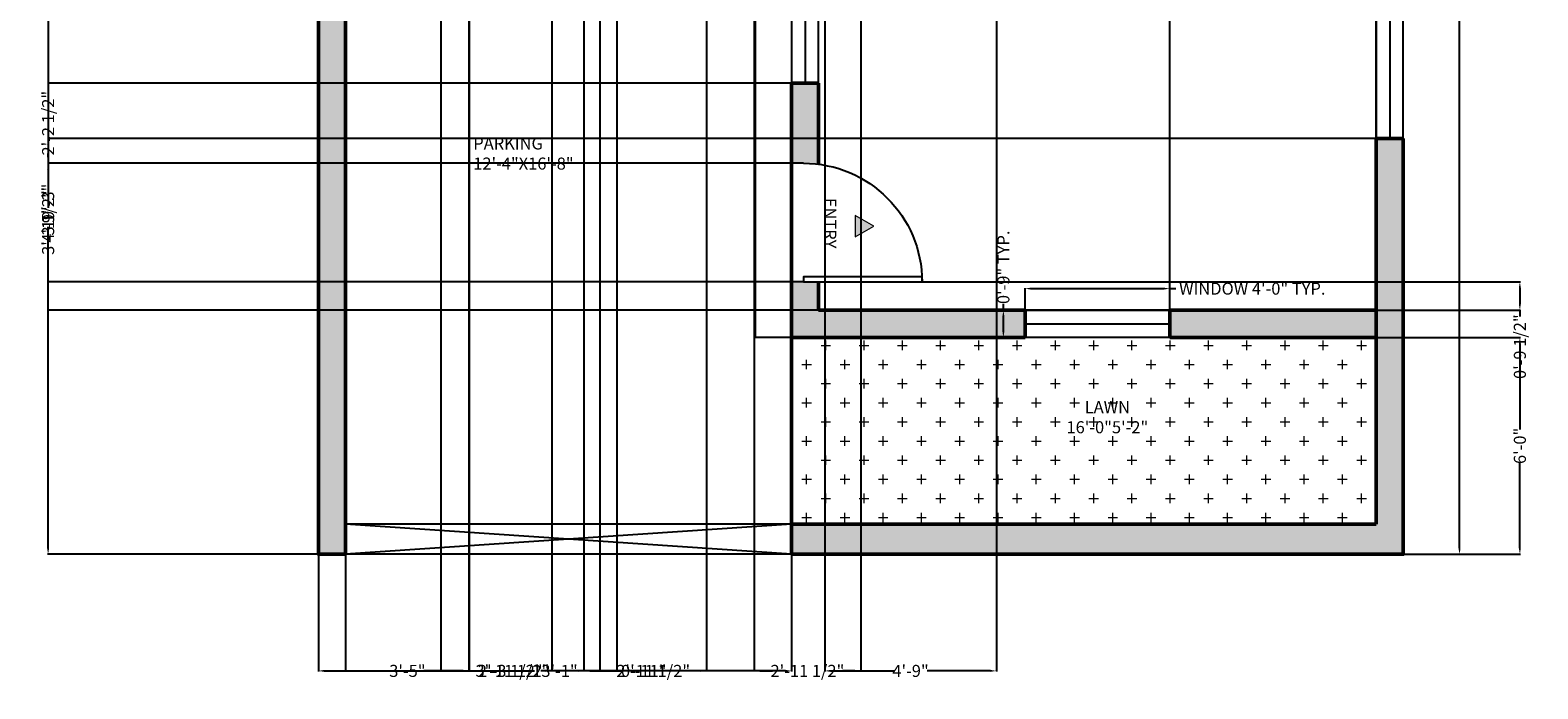
# Model space of a CAD drawing. Units: inches. Extents: x 2430 to 2930, y 1715 to 2575.
# Tile 1 of 4: x 2430 to 2930, y 1715 to 1933. Entities that reach past the tile are written whole.
import ezdxf

# ---------------------------------------------------------------- set-up
doc = ezdxf.new("R2010")
doc.units = ezdxf.units.IN
for name, color, linetype, lineweight in [('A-ANNO-DIMS', 2, 'Continuous', 18), ('A-ANNO-SYMB', 130, 'Continuous', 18), ('A-ANNO-TEXT', 130, 'Continuous', 18), ('A-AREA-IDEN', 130, 'Continuous', 18), ('A-FLOR', 7, 'Continuous', 25), ('A-WALL', 7, 'Continuous', 50), ('A-WALL-PATT', 251, 'Continuous', 13), ('DOOR', 224, 'Continuous', 25), ('L-PLNT-PATT', 116, 'Continuous', 13), ('L-SITE-GATE', 242, 'Continuous', 25), ('win', 170, 'Continuous', 25)]:
    doc.layers.add(name, color=color, linetype=linetype, lineweight=lineweight)
doc.styles.get("Standard").update_dxf_attribs({"font": 'arial.ttf', "height": 4})
doc.dimstyles.get("Standard").update_dxf_attribs({"dimtxt": 4, "dimasz": 2, "dimexe": 0.18, "dimexo": 0.0625, "dimgap": 0.09, "dimtad": 0, "dimzin": 0, "dimdsep": 46, "dimlunit": 3, "dimtxsty": 'Standard', "dimcen": 0.09, "dimadec": 0, "dimazin": 0, "dimtfac": 1, "dimtofl": 0, "dimtmove": 0, "dimatfit": 3, "dimfxl": 1, "dimtolj": 1, "dimtzin": 0, "dimarcsym": 0})

# ---------------------------------------------------------------- blocks, each defined once
blk = doc.blocks.new('*U6')
for p, q in [((0, 0), (0, -100)), ((1000, 0), (1000, -100))]:
    blk.add_line(p, q)
blk.add_lwpolyline([(0, 0), (0, 1000), (43.75, 1000), (43.75, 0)], close=True)
blk.add_arc((0, 0), 1000, 0, 90)
blk = doc.blocks.new('*D12')
at = {"layer": 'A-ANNO-DIMS', "color": 0, "lineweight": -2, "transparency": 16777216}
for p, q in [((2885.68, 2479.45), (2904.48, 2479.45)), ((2904.3, 2477.45), (2904.3, 2122.95)), ((2904.3, 1761.45), (2904.3, 2115.96)), ((2885.68, 1759.45), (2904.48, 1759.45))]:
    blk.add_line(p, q, dxfattribs=at)
at = {"layer": 'A-ANNO-DIMS', "color": 0, "transparency": 16777216}
for points in [[(2903.96, 2477.45), (2904.63, 2477.45), (2904.3, 2479.45)], [(2903.96, 1761.45), (2904.63, 1761.45), (2904.3, 1759.45)]]:
    blk.add_solid(points, dxfattribs=at)
at = {"layer": 'Defpoints', "color": 0, "transparency": 16777216}
for p in [(2885.62, 2479.45), (2885.62, 1759.45), (2904.3, 1759.45)]:
    blk.add_point(p, dxfattribs=at)
at = {"layer": 'A-ANNO-DIMS', "color": 0, "transparency": 16777216, "insert": (2904.3, 2119.45), "char_height": 4, "attachment_point": 5, "rotation": 90}
blk.add_mtext("\\A1;60'", dxfattribs=at)
blk = doc.blocks.new('WIN-48IN')
blk.add_line((0, 4.5), (48, 4.5))
blk.add_lwpolyline([(0, 9), (48, 9), (48, 0), (0, 0)], close=True)
blk = doc.blocks.new('*D17')
at = {"layer": 'A-ANNO-DIMS', "color": 0, "lineweight": -2, "transparency": 16777216}
for p, q in [((2760.12, 1840.52), (2760.12, 1847.83)), ((2762.12, 1847.65), (2806.12, 1847.65)), ((2808.12, 1840.52), (2808.12, 1847.83)), ((2808.12, 1847.65), (2810.12, 1847.65))]:
    blk.add_line(p, q, dxfattribs=at)
at = {"layer": 'A-ANNO-DIMS', "color": 0, "transparency": 16777216}
for points in [[(2762.12, 1847.99), (2762.12, 1847.32), (2760.12, 1847.65)], [(2806.12, 1847.99), (2806.12, 1847.32), (2808.12, 1847.65)]]:
    blk.add_solid(points, dxfattribs=at)
at = {"layer": 'Defpoints', "color": 0, "transparency": 16777216}
for p in [(2808.12, 1847.65), (2760.12, 1840.45), (2808.12, 1840.45)]:
    blk.add_point(p, dxfattribs=at)
at = {"layer": 'A-ANNO-DIMS', "color": 0, "transparency": 16777216, "insert": (2835.52, 1847.65), "char_height": 4, "attachment_point": 5}
blk.add_mtext('\\A1;WINDOW 4\'-0" TYP.', dxfattribs=at)
blk = doc.blocks.new('*D18')
at = {"layer": 'A-ANNO-DIMS', "color": 0, "lineweight": -2, "transparency": 16777216}
for p, q in [((2752.92, 1840.45), (2752.92, 1842.45)), ((2760.06, 1840.45), (2752.74, 1840.45)), ((2752.92, 1833.45), (2752.92, 1838.45)), ((2760.06, 1831.45), (2752.74, 1831.45))]:
    blk.add_line(p, q, dxfattribs=at)
at = {"layer": 'A-ANNO-DIMS', "color": 0, "transparency": 16777216}
for points in [[(2752.59, 1838.45), (2753.25, 1838.45), (2752.92, 1840.45)], [(2752.59, 1833.45), (2753.25, 1833.45), (2752.92, 1831.45)]]:
    blk.add_solid(points, dxfattribs=at)
at = {"layer": 'Defpoints', "color": 0, "transparency": 16777216}
for p in [(2752.92, 1840.45), (2760.12, 1840.45), (2760.12, 1831.45)]:
    blk.add_point(p, dxfattribs=at)
at = {"layer": 'A-ANNO-DIMS', "color": 0, "transparency": 16777216, "insert": (2752.92, 1854.73), "char_height": 4, "attachment_point": 5, "rotation": 90}
blk.add_mtext('\\A1;0\'-9" TYP.', dxfattribs=at)
blk = doc.blocks.new('*D27')
at = {"layer": 'A-ANNO-DIMS', "color": 0, "lineweight": -2, "transparency": 16777216}
for p, q in [((2525.62, 1759.39), (2525.62, 1720.57)), ((2682.62, 1759.39), (2682.62, 1720.57)), ((2527.62, 1720.75), (2597.35, 1720.75)), ((2680.62, 1720.75), (2610.89, 1720.75))]:
    blk.add_line(p, q, dxfattribs=at)
at = {"layer": 'A-ANNO-DIMS', "color": 0, "transparency": 16777216}
for points in [[(2527.62, 1721.09), (2527.62, 1720.42), (2525.62, 1720.75)], [(2680.62, 1721.09), (2680.62, 1720.42), (2682.62, 1720.75)]]:
    blk.add_solid(points, dxfattribs=at)
at = {"layer": 'Defpoints', "color": 0, "transparency": 16777216}
for p in [(2525.62, 1759.45), (2682.62, 1759.45), (2682.62, 1720.75)]:
    blk.add_point(p, dxfattribs=at)
at = {"layer": 'A-ANNO-DIMS', "color": 0, "transparency": 16777216, "insert": (2604.12, 1720.75), "char_height": 4, "attachment_point": 5}
blk.add_mtext('\\A1;13\'-1"', dxfattribs=at)
blk = doc.blocks.new('*D28')
at = {"layer": 'A-ANNO-DIMS', "color": 0, "lineweight": -2, "transparency": 16777216}
for p, q in [((2876.68, 1831.45), (2924.5, 1831.45)), ((2924.32, 1829.45), (2924.32, 1800.87)), ((2924.32, 1761.45), (2924.32, 1790.04)), ((2885.68, 1759.45), (2924.5, 1759.45))]:
    blk.add_line(p, q, dxfattribs=at)
at = {"layer": 'A-ANNO-DIMS', "color": 0, "transparency": 16777216}
for points in [[(2923.99, 1829.45), (2924.65, 1829.45), (2924.32, 1831.45)], [(2923.99, 1761.45), (2924.65, 1761.45), (2924.32, 1759.45)]]:
    blk.add_solid(points, dxfattribs=at)
at = {"layer": 'Defpoints', "color": 0, "transparency": 16777216}
for p in [(2876.62, 1831.45), (2885.62, 1759.45), (2924.32, 1759.45)]:
    blk.add_point(p, dxfattribs=at)
at = {"layer": 'A-ANNO-DIMS', "color": 0, "transparency": 16777216, "insert": (2924.32, 1795.45), "char_height": 4, "attachment_point": 5, "rotation": 90}
blk.add_mtext('\\A1;6\'-0"', dxfattribs=at)
blk = doc.blocks.new('*D29')
at = {"layer": 'A-ANNO-DIMS', "color": 0, "lineweight": -2, "transparency": 16777216}
for p, q in [((2682.56, 1889.27), (2435.74, 1889.27)), ((2435.92, 1887.27), (2435.92, 1879.65)), ((2435.92, 1851.9), (2435.92, 1859.52)), ((2682.56, 1849.9), (2435.74, 1849.9))]:
    blk.add_line(p, q, dxfattribs=at)
at = {"layer": 'A-ANNO-DIMS', "color": 0, "transparency": 16777216}
for points in [[(2435.59, 1887.27), (2436.25, 1887.27), (2435.92, 1889.27)], [(2435.59, 1851.9), (2436.25, 1851.9), (2435.92, 1849.9)]]:
    blk.add_solid(points, dxfattribs=at)
at = {"layer": 'Defpoints', "color": 0, "transparency": 16777216}
for p in [(2435.92, 1889.27), (2682.62, 1889.27), (2682.62, 1849.9)]:
    blk.add_point(p, dxfattribs=at)
at = {"layer": 'A-ANNO-DIMS', "color": 0, "transparency": 16777216, "insert": (2435.92, 1869.58), "char_height": 4, "attachment_point": 5, "rotation": 90}
blk.add_mtext('\\A1;3\'-3 1/2"', dxfattribs=at)
blk = doc.blocks.new('*D30')
at = {"layer": 'A-ANNO-DIMS', "color": 0, "lineweight": -2, "transparency": 16777216}
for p, q in [((2534.62, 2470.39), (2534.62, 1720.57)), ((2575.68, 2470.39), (2575.68, 1720.57)), ((2536.62, 1720.75), (2549.75, 1720.75)), ((2573.68, 1720.75), (2560.56, 1720.75))]:
    blk.add_line(p, q, dxfattribs=at)
at = {"layer": 'A-ANNO-DIMS', "color": 0, "transparency": 16777216}
for points in [[(2536.62, 1721.09), (2536.62, 1720.42), (2534.62, 1720.75)], [(2573.68, 1721.09), (2573.68, 1720.42), (2575.68, 1720.75)]]:
    blk.add_solid(points, dxfattribs=at)
at = {"layer": 'Defpoints', "color": 0, "transparency": 16777216}
for p in [(2534.62, 2470.45), (2575.68, 2470.45), (2575.68, 1720.75)]:
    blk.add_point(p, dxfattribs=at)
at = {"layer": 'A-ANNO-DIMS', "color": 0, "transparency": 16777216, "insert": (2555.15, 1720.75), "char_height": 4, "attachment_point": 5}
blk.add_mtext('\\A1;3\'-5"', dxfattribs=at)
blk = doc.blocks.new('*D34')
at = {"layer": 'A-ANNO-DIMS', "color": 0, "lineweight": -2, "transparency": 16777216}
for p, q in [((2525.56, 1990.45), (2435.74, 1990.45)), ((2435.92, 1988.45), (2435.92, 1881.72)), ((2435.92, 1761.45), (2435.92, 1868.18)), ((2525.56, 1759.45), (2435.74, 1759.45))]:
    blk.add_line(p, q, dxfattribs=at)
at = {"layer": 'A-ANNO-DIMS', "color": 0, "transparency": 16777216}
for points in [[(2435.59, 1988.45), (2436.25, 1988.45), (2435.92, 1990.45)], [(2435.59, 1761.45), (2436.25, 1761.45), (2435.92, 1759.45)]]:
    blk.add_solid(points, dxfattribs=at)
at = {"layer": 'Defpoints', "color": 0, "transparency": 16777216}
for p in [(2435.92, 1990.45), (2525.62, 1990.45), (2525.62, 1759.45)]:
    blk.add_point(p, dxfattribs=at)
at = {"layer": 'A-ANNO-DIMS', "color": 0, "transparency": 16777216, "insert": (2435.92, 1874.95), "char_height": 4, "attachment_point": 5, "rotation": 90}
blk.add_mtext('\\A1;19\'-3"', dxfattribs=at)
blk = doc.blocks.new('*D38')
at = {"layer": 'A-ANNO-DIMS', "color": 0, "lineweight": -2, "transparency": 16777216}
for p, q in [((2876.56, 1897.45), (2435.74, 1897.45)), ((2435.92, 1895.45), (2435.92, 1874.44)), ((2435.92, 1842.45), (2435.92, 1863.47)), ((2876.56, 1840.45), (2435.74, 1840.45))]:
    blk.add_line(p, q, dxfattribs=at)
at = {"layer": 'A-ANNO-DIMS', "color": 0, "transparency": 16777216}
for points in [[(2435.59, 1895.45), (2436.25, 1895.45), (2435.92, 1897.45)], [(2435.59, 1842.45), (2436.25, 1842.45), (2435.92, 1840.45)]]:
    blk.add_solid(points, dxfattribs=at)
at = {"layer": 'Defpoints', "color": 0, "transparency": 16777216}
for p in [(2876.62, 1897.45), (2435.92, 1840.45), (2876.62, 1840.45)]:
    blk.add_point(p, dxfattribs=at)
at = {"layer": 'A-ANNO-DIMS', "color": 0, "transparency": 16777216, "insert": (2435.92, 1868.95), "char_height": 4, "attachment_point": 5, "rotation": 90}
blk.add_mtext('\\A1;4\'-9"', dxfattribs=at)
blk = doc.blocks.new('*D39')
at = {"layer": 'A-ANNO-DIMS', "color": 0, "lineweight": -2, "transparency": 16777216}
for p, q in [((2808.12, 1840.52), (2808.12, 2569.33)), ((2810.12, 2569.15), (2832.3, 2569.15)), ((2874.62, 2569.15), (2852.44, 2569.15)), ((2876.62, 1840.52), (2876.62, 2569.33))]:
    blk.add_line(p, q, dxfattribs=at)
at = {"layer": 'A-ANNO-DIMS', "color": 0, "transparency": 16777216}
for points in [[(2810.12, 2569.49), (2810.12, 2568.82), (2808.12, 2569.15)], [(2874.62, 2569.49), (2874.62, 2568.82), (2876.62, 2569.15)]]:
    blk.add_solid(points, dxfattribs=at)
at = {"layer": 'Defpoints', "color": 0, "transparency": 16777216}
for p in [(2876.62, 2569.15), (2808.12, 1840.45), (2876.62, 1840.45)]:
    blk.add_point(p, dxfattribs=at)
at = {"layer": 'A-ANNO-DIMS', "color": 0, "transparency": 16777216, "insert": (2842.37, 2569.15), "char_height": 4, "attachment_point": 5}
blk.add_mtext('\\A1;5\'-8 1/2"', dxfattribs=at)
blk = doc.blocks.new('*D41')
at = {"layer": 'A-ANNO-DIMS', "color": 0, "lineweight": -2, "transparency": 16777216}
for p, q in [((2693.62, 2062.39), (2693.62, 1720.57)), ((2750.62, 2056.39), (2750.62, 1720.57)), ((2695.62, 1720.75), (2716.63, 1720.75)), ((2748.62, 1720.75), (2727.61, 1720.75))]:
    blk.add_line(p, q, dxfattribs=at)
at = {"layer": 'A-ANNO-DIMS', "color": 0, "transparency": 16777216}
for points in [[(2695.62, 1721.09), (2695.62, 1720.42), (2693.62, 1720.75)], [(2748.62, 1721.09), (2748.62, 1720.42), (2750.62, 1720.75)]]:
    blk.add_solid(points, dxfattribs=at)
at = {"layer": 'Defpoints', "color": 0, "transparency": 16777216}
for p in [(2693.62, 2062.45), (2750.62, 2056.45), (2750.62, 1720.75)]:
    blk.add_point(p, dxfattribs=at)
at = {"layer": 'A-ANNO-DIMS', "color": 0, "transparency": 16777216, "insert": (2722.12, 1720.75), "char_height": 4, "attachment_point": 5}
blk.add_mtext('\\A1;4\'-9"', dxfattribs=at)
blk = doc.blocks.new('*D44')
at = {"layer": 'A-ANNO-DIMS', "color": 0, "lineweight": -2, "transparency": 16777216}
for p, q in [((2670.19, 2218.39), (2670.19, 1720.57)), ((2705.62, 2218.39), (2705.62, 1720.57)), ((2672.19, 1720.75), (2676.25, 1720.75)), ((2703.62, 1720.75), (2699.56, 1720.75))]:
    blk.add_line(p, q, dxfattribs=at)
at = {"layer": 'A-ANNO-DIMS', "color": 0, "transparency": 16777216}
for points in [[(2672.19, 1721.09), (2672.19, 1720.42), (2670.19, 1720.75)], [(2703.62, 1721.09), (2703.62, 1720.42), (2705.62, 1720.75)]]:
    blk.add_solid(points, dxfattribs=at)
at = {"layer": 'Defpoints', "color": 0, "transparency": 16777216}
for p in [(2670.19, 2218.45), (2705.62, 2218.45), (2670.19, 1720.75)]:
    blk.add_point(p, dxfattribs=at)
at = {"layer": 'A-ANNO-DIMS', "color": 0, "transparency": 16777216, "insert": (2687.9, 1720.75), "char_height": 4, "attachment_point": 5}
blk.add_mtext('\\A1;2\'-11 1/2"', dxfattribs=at)
blk = doc.blocks.new('*D45')
at = {"layer": 'A-ANNO-DIMS', "color": 0, "lineweight": -2, "transparency": 16777216}
for p, q in [((2619.01, 2380.39), (2619.01, 1720.57)), ((2654.44, 2380.39), (2654.44, 1720.57)), ((2621.01, 1720.75), (2625.07, 1720.75)), ((2652.44, 1720.75), (2648.38, 1720.75))]:
    blk.add_line(p, q, dxfattribs=at)
at = {"layer": 'A-ANNO-DIMS', "color": 0, "transparency": 16777216}
for points in [[(2621.01, 1721.09), (2621.01, 1720.42), (2619.01, 1720.75)], [(2652.44, 1721.09), (2652.44, 1720.42), (2654.44, 1720.75)]]:
    blk.add_solid(points, dxfattribs=at)
at = {"layer": 'Defpoints', "color": 0, "transparency": 16777216}
for p in [(2619.01, 2380.45), (2654.44, 2380.45), (2654.44, 1720.75)]:
    blk.add_point(p, dxfattribs=at)
at = {"layer": 'A-ANNO-DIMS', "color": 0, "transparency": 16777216, "insert": (2636.72, 1720.75), "char_height": 4, "attachment_point": 5}
blk.add_mtext('\\A1;2\'-11 1/2"', dxfattribs=at)
blk = doc.blocks.new('*D46')
at = {"layer": 'A-ANNO-DIMS', "color": 0, "lineweight": -2, "transparency": 16777216}
for p, q in [((2575.5, 2380.39), (2575.5, 1720.57)), ((2603.06, 2380.39), (2603.06, 1720.57)), ((2577.5, 1720.75), (2579.18, 1720.75)), ((2601.06, 1720.75), (2599.38, 1720.75))]:
    blk.add_line(p, q, dxfattribs=at)
at = {"layer": 'A-ANNO-DIMS', "color": 0, "transparency": 16777216}
for points in [[(2577.5, 1721.09), (2577.5, 1720.42), (2575.5, 1720.75)], [(2601.06, 1721.09), (2601.06, 1720.42), (2603.06, 1720.75)]]:
    blk.add_solid(points, dxfattribs=at)
at = {"layer": 'Defpoints', "color": 0, "transparency": 16777216}
for p in [(2575.5, 2380.45), (2603.06, 2380.45), (2603.06, 1720.75)]:
    blk.add_point(p, dxfattribs=at)
at = {"layer": 'A-ANNO-DIMS', "color": 0, "transparency": 16777216, "insert": (2589.28, 1720.75), "char_height": 4, "attachment_point": 5}
blk.add_mtext('\\A1;2\'-3 1/2"', dxfattribs=at)
blk = doc.blocks.new('*D47')
at = {"layer": 'A-ANNO-DIMS', "color": 0, "lineweight": -2, "transparency": 16777216}
for p, q in [((2682.56, 1915.89), (2435.74, 1915.89)), ((2435.92, 1913.89), (2435.92, 1912.68)), ((2435.92, 1891.27), (2435.92, 1892.48)), ((2682.56, 1889.27), (2435.74, 1889.27))]:
    blk.add_line(p, q, dxfattribs=at)
at = {"layer": 'A-ANNO-DIMS', "color": 0, "transparency": 16777216}
for points in [[(2435.59, 1913.89), (2436.25, 1913.89), (2435.92, 1915.89)], [(2435.59, 1891.27), (2436.25, 1891.27), (2435.92, 1889.27)]]:
    blk.add_solid(points, dxfattribs=at)
at = {"layer": 'Defpoints', "color": 0, "transparency": 16777216}
for p in [(2435.92, 1915.89), (2682.62, 1915.89), (2682.62, 1889.27)]:
    blk.add_point(p, dxfattribs=at)
at = {"layer": 'A-ANNO-DIMS', "color": 0, "transparency": 16777216, "insert": (2435.92, 1902.58), "char_height": 4, "attachment_point": 5, "rotation": 90}
blk.add_mtext('\\A1;2\'-2 1/2"', dxfattribs=at)
blk = doc.blocks.new('*D48')
at = {"layer": 'A-ANNO-DIMS', "color": 0, "lineweight": -2, "transparency": 16777216}
for p, q in [((2691.68, 1849.9), (2924.5, 1849.9)), ((2924.32, 1847.9), (2924.32, 1842.45)), ((2691.68, 1840.45), (2924.5, 1840.45)), ((2924.32, 1840.45), (2924.32, 1838.45))]:
    blk.add_line(p, q, dxfattribs=at)
at = {"layer": 'A-ANNO-DIMS', "color": 0, "transparency": 16777216}
for points in [[(2923.99, 1847.9), (2924.65, 1847.9), (2924.32, 1849.9)], [(2923.99, 1842.45), (2924.65, 1842.45), (2924.32, 1840.45)]]:
    blk.add_solid(points, dxfattribs=at)
at = {"layer": 'Defpoints', "color": 0, "transparency": 16777216}
for p in [(2691.62, 1849.9), (2691.62, 1840.45), (2924.32, 1840.45)]:
    blk.add_point(p, dxfattribs=at)
at = {"layer": 'A-ANNO-DIMS', "color": 0, "transparency": 16777216, "insert": (2924.32, 1828.39), "char_height": 4, "attachment_point": 5, "rotation": 90}
blk.add_mtext('\\A1;0\'-9 1/2"', dxfattribs=at)
blk = doc.blocks.new('*D51')
at = {"layer": 'A-ANNO-DIMS', "color": 0, "lineweight": -2, "transparency": 16777216}
for p, q in [((2566.24, 2197.83), (2566.24, 1720.57)), ((2613.75, 2197.83), (2613.75, 1720.57)), ((2568.24, 1720.75), (2578.38, 1720.75)), ((2611.75, 1720.75), (2601.62, 1720.75))]:
    blk.add_line(p, q, dxfattribs=at)
at = {"layer": 'A-ANNO-DIMS', "color": 0, "transparency": 16777216}
for points in [[(2568.24, 1721.09), (2568.24, 1720.42), (2566.24, 1720.75)], [(2611.75, 1721.09), (2611.75, 1720.42), (2613.75, 1720.75)]]:
    blk.add_solid(points, dxfattribs=at)
at = {"layer": 'Defpoints', "color": 0, "transparency": 16777216}
for p in [(2566.24, 2197.89), (2613.75, 2197.89), (2613.75, 1720.75)]:
    blk.add_point(p, dxfattribs=at)
at = {"layer": 'A-ANNO-DIMS', "color": 0, "transparency": 16777216, "insert": (2590, 1720.75), "char_height": 4, "attachment_point": 5}
blk.add_mtext('\\A1;3\'-11 1/2"', dxfattribs=at)
blk = doc.blocks.new('*D53')
at = {"layer": 'A-ANNO-DIMS', "color": 0, "lineweight": -2, "transparency": 16777216}
for p, q in [((2613.75, 2197.83), (2613.75, 1720.57)), ((2624.62, 2194.39), (2624.62, 1720.57)), ((2615.75, 1720.75), (2622.62, 1720.75)), ((2624.62, 1720.75), (2626.62, 1720.75))]:
    blk.add_line(p, q, dxfattribs=at)
at = {"layer": 'A-ANNO-DIMS', "color": 0, "transparency": 16777216}
for points in [[(2615.75, 1721.09), (2615.75, 1720.42), (2613.75, 1720.75)], [(2622.62, 1721.09), (2622.62, 1720.42), (2624.62, 1720.75)]]:
    blk.add_solid(points, dxfattribs=at)
at = {"layer": 'Defpoints', "color": 0, "transparency": 16777216}
for p in [(2613.75, 2197.89), (2624.62, 2194.45), (2624.62, 1720.75)]:
    blk.add_point(p, dxfattribs=at)
at = {"layer": 'A-ANNO-DIMS', "color": 0, "transparency": 16777216, "insert": (2633.58, 1720.75), "char_height": 4, "attachment_point": 5}
blk.add_mtext('\\A1;0\'-11"', dxfattribs=at)

msp = doc.modelspace()

# ---------------------------------------------------------------- hatches: boundary and pattern name
at = {"layer": 'A-ANNO-SYMB'}
h = msp.add_hatch(color=256, dxfattribs=at)
h.dxf.hatch_style = 1
h.paths.add_polyline_path([(2709.881, 1868.357), (2703.752, 1871.895), (2703.752, 1864.818)])
at = {"layer": 'A-WALL-PATT'}
h = msp.add_hatch(color=256, dxfattribs=at)
h.dxf.hatch_style = 1
h.paths.add_polyline_path([(2885.621, 1897.453), (2876.621, 1897.453), (2876.621, 1769.453), (2682.621, 1769.453), (2682.621, 1759.453), (2885.621, 1759.453)])
h.paths.add_polyline_path([(2885.621, 2020.453), (2876.621, 2020.453), (2876.621, 1945.453), (2885.621, 1945.453)])
h.paths.add_polyline_path([(2876.621, 1840.453), (2808.121, 1840.453), (2808.121, 1831.453), (2876.621, 1831.453)], flags=17)
h.paths.add_polyline_path([(2760.121, 1840.453), (2691.621, 1840.453), (2691.621, 1849.896), (2686.558, 1849.896), (2682.621, 1849.896), (2682.621, 1831.453), (2760.121, 1831.453)], flags=17)
h.paths.add_polyline_path([(2691.621, 1915.889), (2682.621, 1915.889), (2682.621, 1889.266), (2686.558, 1889.266, -0.0322505), (2691.621, 1888.939)])
h.paths.add_polyline_path([(2691.621, 2056.453), (2693.621, 2056.453), (2693.621, 2062.453), (2682.621, 2062.453), (2677.568, 2062.453), (2677.568, 2057.39), (2677.568, 2053.453), (2682.621, 2053.453), (2682.621, 1975.453), (2673.244, 1975.453), (2673.244, 1970.39), (2673.244, 1966.453), (2682.621, 1966.453), (2682.621, 1963.889), (2691.621, 1963.889)])
h.paths.add_polyline_path([(2641.748, 1970.39, -0.0403846), (2642.158, 1975.453), (2534.621, 1975.453), (2534.621, 1966.453), (2641.748, 1966.453)])
h.paths.add_polyline_path([(2534.621, 1990.453), (2525.621, 1990.453), (2525.621, 1759.453), (2534.621, 1759.453)])
at = {"layer": 'L-PLNT-PATT'}
h = msp.add_hatch(dxfattribs=at)
h.set_pattern_fill('CROSS', color=256)
h.paths.add_polyline_path([(2876.621, 1831.453), (2808.121, 1831.453), (2760.121, 1831.453), (2682.621, 1831.453), (2682.621, 1769.453), (2876.621, 1769.453)])

# ---------------------------------------------------------------- linework, layer by layer
at = {"layer": 'A-ANNO-SYMB'}
msp.add_lwpolyline([(2709.881, 1868.357), (2703.752, 1871.895), (2703.752, 1864.818)], close=True, dxfattribs=at)
at = {"layer": 'A-FLOR'}
for p, q in [((2670.621, 1831.453), (2670.621, 1954.453)), ((2682.621, 1831.453), (2670.621, 1831.453))]:
    msp.add_line(p, q, dxfattribs=at)
at = {"layer": 'A-WALL'}
for p, q in [((2534.621, 1759.453), (2534.621, 1990.453)), ((2682.621, 1759.453), (2682.621, 1915.889)), ((2682.621, 1915.889), (2691.621, 1915.889)), ((2691.621, 1888.939), (2691.621, 1915.889)), ((2876.621, 1897.453), (2885.621, 1897.453)), ((2876.621, 1897.453), (2876.621, 1769.453)), ((2691.621, 1840.453), (2691.621, 1849.896)), ((2691.621, 1840.453), (2760.121, 1840.453)), ((2760.121, 1840.453), (2760.121, 1831.453)), ((2808.121, 1840.453), (2808.121, 1831.453)), ((2808.121, 1840.453), (2876.621, 1840.453)), ((2682.621, 1831.453), (2760.121, 1831.453)), ((2808.121, 1831.453), (2876.621, 1831.453)), ((2682.621, 1769.453), (2876.621, 1769.453))]:
    msp.add_line(p, q, dxfattribs=at)
for points in [[(2534.621, 1759.453), (2525.621, 1759.453), (2525.621, 1990.453)], [(2885.621, 1897.453), (2885.621, 1759.453), (2682.621, 1759.453)]]:
    msp.add_lwpolyline(points, dxfattribs=at)
at = {"layer": 'L-SITE-GATE'}
for p, q in [((2682.621, 1759.453), (2534.621, 1769.453)), ((2682.621, 1769.453), (2534.621, 1759.453)), ((2682.621, 1769.453), (2534.621, 1769.453)), ((2682.621, 1759.453), (2534.621, 1759.453))]:
    msp.add_line(p, q, dxfattribs=at)

# ---------------------------------------------------------------- block references
at = {"layer": 'DOOR', "xscale": -0.0393700787401575, "yscale": 0.0393700787401575, "zscale": 0.0393700787401575, "rotation": 270}
msp.add_blockref('*U6', (2686.558, 1849.896), dxfattribs=at)
at = {"layer": 'win', "extrusion": (0, 0, -1), "zscale": -1}
for p, rotation in [((-2691.621, 1963.89), 270.0000000000003), ((-2885.621, 1945.453), 270.0000000000005)]:
    msp.add_blockref('WIN-48IN', p, dxfattribs=dict(at, rotation=rotation))
at = {"layer": 'win'}
msp.add_blockref('WIN-48IN', (2760.121, 1831.453), dxfattribs=at)

# ---------------------------------------------------------------- texts
at = {"layer": 'A-ANNO-TEXT', "insert": (2697.502, 1877.784), "char_height": 4, "attachment_point": 1, "rotation": 270}
msp.add_mtext_dynamic_manual_height_columns('ENTRY', width=13.10191, gutter_width=20, heights=[0], dxfattribs=at)
at = {"layer": 'A-AREA-IDEN', "char_height": 4, "attachment_point": 1}
for s, width, insert in [('PARKING\\P12\'-4"X16\'-8"', 31.75805, (2577.014, 1897.834)), ('\\pxqc;LAWN\\P16\'-0"5\'-2"', 47.75462, (2763.562, 1810.304))]:
    msp.add_mtext_dynamic_manual_height_columns(s, width=width, gutter_width=20, heights=[0], dxfattribs=dict(at, insert=insert))

# ---------------------------------------------------------------- dimensions: what is measured, and where the dimension line sits
at = {"layer": 'A-ANNO-DIMS'}
for base, p1, p2, picture, middle in [((2876.621, 2569.153), (2808.121, 1840.453), (2876.621, 1840.453), '*D39', (2842.371, 2569.153)), ((2575.684, 1720.753), (2534.621, 2470.453), (2575.684, 2470.453), '*D30', (2555.153, 1720.753)), ((2603.056, 1720.753), (2575.497, 2380.453), (2603.056, 2380.453), '*D46', (2589.277, 1720.753)), ((2654.438, 1720.753), (2619.005, 2380.453), (2654.438, 2380.453), '*D45', (2636.722, 1720.753)), ((2670.188, 1720.753), (2705.621, 2218.453), (2670.188, 2218.453), '*D44', (2687.905, 1720.753)), ((2613.749, 1720.753), (2566.245, 2197.895), (2613.749, 2197.895), '*D51', (2589.997, 1720.753)), ((2624.621, 1720.753), (2613.749, 2197.895), (2624.621, 2194.453), '*D53', (2633.582, 1720.753)), ((2750.621, 1720.753), (2693.621, 2062.453), (2750.621, 2056.453), '*D41', (2722.121, 1720.753)), ((2682.621, 1720.753), (2525.621, 1759.453), (2682.621, 1759.453), '*D27', (2604.121, 1720.753))]:
    dim = msp.add_linear_dim(base=base, p1=p1, p2=p2, dimstyle='Standard', override={"dimdec": 1, "dimlfac": 1, "dimrnd": 0, "dimzin": 1, "dimdsep": 46, "dimlunit": 4, "dimfrac": 2}, dxfattribs=at)
    dim.commit()
    dim.dimension.update_dxf_attribs({"geometry": picture, "text_midpoint": middle})
for base, p1, p2, override, picture, middle in [((2904.296, 1759.453), (2885.621, 2479.453), (2885.621, 1759.453), {"dimclrd": 0, "dimclre": 0, "dimclrt": 0}, '*D12', (2904.296, 2119.453)), ((2435.921, 1990.453), (2525.621, 1759.453), (2525.621, 1990.453), {"dimdec": 1, "dimlfac": 1, "dimrnd": 0, "dimzin": 1, "dimdsep": 46, "dimlunit": 4, "dimfrac": 2}, '*D34', (2435.921, 1874.953)), ((2435.921, 1915.889), (2682.621, 1889.266), (2682.621, 1915.889), {"dimdec": 1, "dimlfac": 1, "dimrnd": 0, "dimzin": 1, "dimdsep": 46, "dimlunit": 4, "dimfrac": 2}, '*D47', (2435.921, 1902.578)), ((2435.921, 1840.453), (2876.621, 1897.453), (2876.621, 1840.453), {"dimdec": 1, "dimlfac": 1, "dimrnd": 0, "dimzin": 1, "dimdsep": 46, "dimlunit": 4, "dimfrac": 2}, '*D38', (2435.921, 1868.953)), ((2435.921, 1889.266), (2682.621, 1849.896), (2682.621, 1889.266), {"dimdec": 1, "dimlfac": 1, "dimrnd": 0, "dimzin": 1, "dimdsep": 46, "dimlunit": 4, "dimfrac": 2}, '*D29', (2435.921, 1869.581)), ((2924.321, 1840.453), (2691.621, 1849.896), (2691.621, 1840.453), {"dimdec": 1, "dimlfac": 1, "dimrnd": 0, "dimzin": 1, "dimdsep": 46, "dimlunit": 4, "dimfrac": 2}, '*D48', (2924.321, 1828.386)), ((2924.321, 1759.453), (2876.621, 1831.453), (2885.621, 1759.453), {"dimdec": 1, "dimlfac": 1, "dimrnd": 0, "dimzin": 1, "dimdsep": 46, "dimlunit": 4, "dimfrac": 2}, '*D28', (2924.321, 1795.453))]:
    dim = msp.add_linear_dim(base=base, p1=p1, p2=p2, angle=90, dimstyle='Standard', override=override, dxfattribs=at)
    dim.commit()
    dim.dimension.update_dxf_attribs({"geometry": picture, "text_midpoint": middle})
dim = msp.add_linear_dim(base=(2752.921, 1840.453), p1=(2760.121, 1831.453), p2=(2760.121, 1840.453), angle=90, text='<> TYP.', dimstyle='Standard', override={"dimdec": 1, "dimlfac": 1, "dimrnd": 0, "dimzin": 1, "dimdsep": 46, "dimlunit": 4, "dimfrac": 2}, dxfattribs=at)
dim.commit()
dim.dimension.update_dxf_attribs({"geometry": '*D18', "text_midpoint": (2752.921, 1854.734)})
dim = msp.add_linear_dim(base=(2808.121, 1847.653), p1=(2760.121, 1840.453), p2=(2808.121, 1840.453), text='WINDOW <> TYP.', dimstyle='Standard', override={"dimdec": 1, "dimlfac": 1, "dimrnd": 0, "dimzin": 1, "dimdsep": 46, "dimlunit": 4, "dimfrac": 2}, dxfattribs=at)
dim.commit()
dim.dimension.update_dxf_attribs({"geometry": '*D17', "text_midpoint": (2835.52, 1847.653)})

doc.saveas('drawing.dxf')
